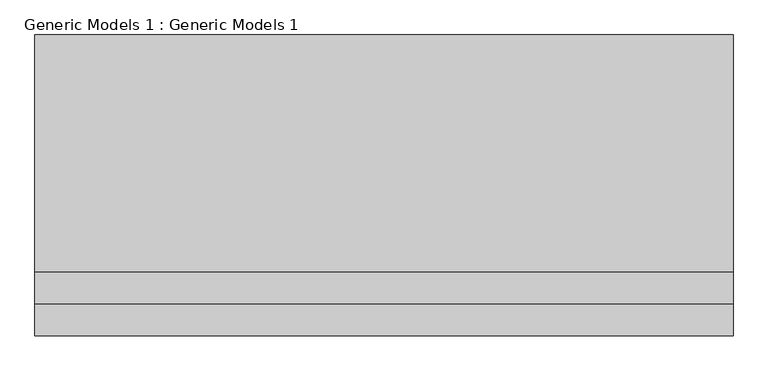
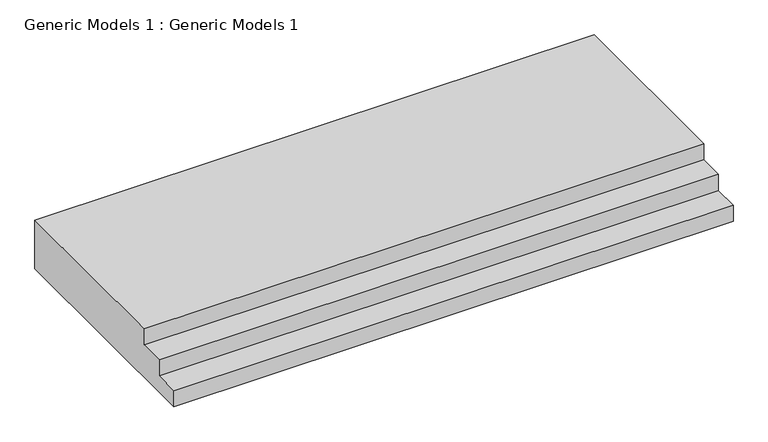
"""IFC4 building model written with IfcOpenShell, lengths in millimetres: proxy geometry, Generic Models 1 : Generic Models 1."""

from ifc_helpers import new_model, si_unit, frame, origin, place, context, project, spatial, polyline, outline, extrude, source, transform, mapped, element, save


def generic_models_1_generic_models_1_6f844308(model_context):
    return source(origin(), model_context, "Body", "SweptSolid", [
        extrude(outline(polyline([(-15025.1944793, 50.8), (-14720.3944793, 50.8), (-14720.3944793, 254.0), (-14415.5944793, 254.0), (-14415.5944793, 457.2), (-12159.6477877, 457.2), (-12159.6477877, -152.4), (-15025.1944793, -152.4), (-15025.1944793, 50.8)])), frame((-8216.9175664, 0.0, 0.0), z_axis=(1.0, 0.0, 0.0), x_axis=(0.0, 1.0, 0.0)), (0.0, 0.0, 1.0), 6653.5772616),
    ])


if __name__ == "__main__":
    model = new_model("IFC4")
    model_context = context("Model", 3, world=origin())
    ifc_project = project(units=[si_unit("LENGTHUNIT", "METRE", prefix="MILLI")], contexts=[model_context])
    site = spatial("IfcSite", under=ifc_project)
    building = spatial("IfcBuilding", under=site)
    placement = place(None, origin())
    generic_models_1_generic_models_1_shape = generic_models_1_generic_models_1_6f844308(model_context)
    element("IfcBuildingElementProxy", 1, Name="Generic Models 1 : Generic Models 1", ObjectType="Generic Models 1 : Generic Models 1", at=placement, inside=building, context=model_context, shape_type="MappedRepresentation", body=[
        mapped(generic_models_1_generic_models_1_shape, transform((0.0, 0.0, 0.0), x_axis=(1.0, 0.0, 0.0), y_axis=(0.0, 1.0, 0.0), z_axis=(0.0, 0.0, 1.0))),
    ])
    save(model, "model.ifc")

# Revit data of these elements
# Element 1 (IfcBuildingElementProxy, "Generic Models 1 : Generic Models 1")
#   Materials on its faces: "Laminate, Ivory, Matte"
# Materials
#   "Laminate, Ivory, Matte": class "Plastic", colour RGB 247 247 239, transparency 0, Description = "Plastic Laminate - Ivory, Matte", Cost = 0
